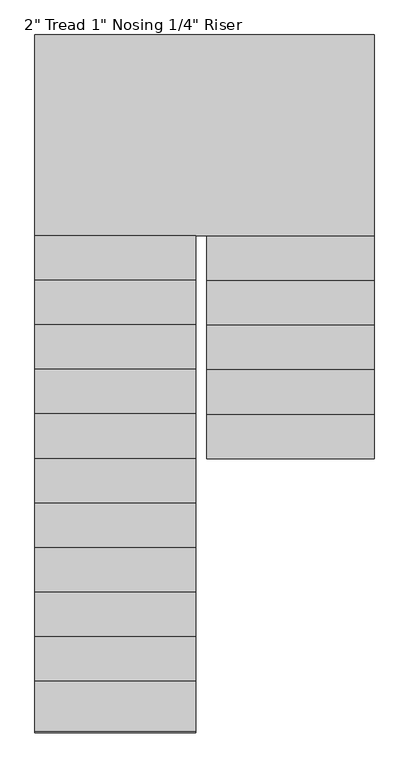
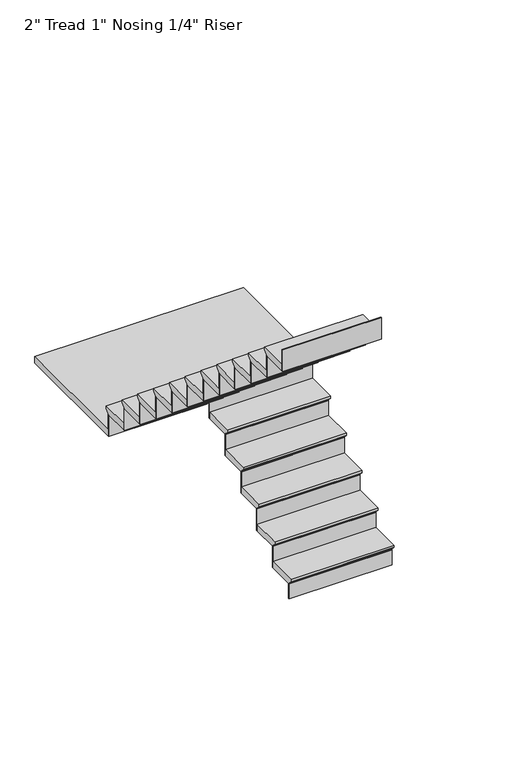
"""IFC4 building model written with IfcOpenShell, lengths in millimetres: stair flight geometry."""

from ifc_helpers import new_model, si_unit, origin, place, context, project, spatial, faceted_brep, source, transform, mapped, element, save


def stair_flight_b92ce0aa(model_context):
    return source(origin(), model_context, "Body", "Brep", [
        faceted_brep([(-3749.597125, 2714.6319226, 12189.8833333), (-3749.597125, 2714.6319226, 12208.9333333), (-4512.2136682, 2714.6319226, 12208.9333333), (-4512.2136682, 2714.6319226, 12189.8833333), (-3749.597125, 2740.0319226, 12164.4833333), (-4512.2136682, 2740.0319226, 12164.4833333), (-3749.597125, 2943.2319226, 12208.9333333), (-4512.2136682, 2943.2319226, 12208.9333333), (-4512.2136682, 2740.0319226, 12158.1333333), (-4512.2136682, 2943.2319226, 12158.1333333), (-3749.597125, 2943.2319226, 12158.1333333), (-3749.597125, 2740.0319226, 12158.1333333)], [[[0, 1, 2, 3]], [[4, 0, 3, 5]], [[2, 1, 6, 7]], [[8, 9, 10, 11]], [[2, 7, 9, 8, 5, 3]], [[8, 11, 4, 5]], [[6, 1, 0, 4, 11, 10]], [[7, 6, 10, 9]]]),
        faceted_brep([(-3749.597125, 2740.0319226, 12158.1333333), (-3749.597125, 2740.0319226, 12039.6), (-3749.597125, 2746.3819226, 12039.6), (-3749.597125, 2746.3819226, 12158.1333333), (-4512.2136682, 2740.0319226, 12158.1333333), (-4512.2136682, 2746.3819226, 12158.1333333), (-4512.2136682, 2746.3819226, 12039.6), (-4512.2136682, 2740.0319226, 12039.6)], [[[0, 1, 2, 3]], [[4, 5, 6, 7]], [[1, 0, 4, 7]], [[2, 1, 7, 6]], [[3, 2, 6, 5]], [[0, 3, 5, 4]]]),
        faceted_brep([(-3749.597125, 2943.2319226, 12327.4666667), (-3749.597125, 2943.2319226, 12158.1333333), (-3749.597125, 2949.5819226, 12158.1333333), (-3749.597125, 2949.5819226, 12327.4666667), (-4512.2136682, 2943.2319226, 12327.4666667), (-4512.2136682, 2949.5819226, 12327.4666667), (-4512.2136682, 2949.5819226, 12158.1333333), (-4512.2136682, 2943.2319226, 12158.1333333)], [[[0, 1, 2, 3]], [[4, 5, 6, 7]], [[1, 0, 4, 7]], [[2, 1, 7, 6]], [[3, 2, 6, 5]], [[0, 3, 5, 4]]]),
        faceted_brep([(-4512.2136682, 2917.8319226, 12378.2666667), (-3749.597125, 2917.8319226, 12378.2666667), (-3749.597125, 3146.4319226, 12378.2666667), (-4512.2136682, 3146.4319226, 12378.2666667), (-4512.2136682, 2943.2319226, 12327.4666667), (-4512.2136682, 3146.4319226, 12327.4666667), (-3749.597125, 3146.4319226, 12327.4666667), (-3749.597125, 2943.2319226, 12327.4666667), (-4512.2136682, 2943.2319226, 12333.8166667), (-4512.2136682, 2917.8319226, 12359.2166667), (-3749.597125, 2943.2319226, 12333.8166667), (-3749.597125, 2917.8319226, 12359.2166667)], [[[0, 1, 2, 3]], [[4, 5, 6, 7]], [[0, 3, 5, 4, 8, 9]], [[4, 7, 10, 8]], [[2, 1, 11, 10, 7, 6]], [[3, 2, 6, 5]], [[11, 1, 0, 9]], [[10, 11, 9, 8]]]),
        faceted_brep([(-3749.597125, 3146.4319226, 12496.8), (-3749.597125, 3146.4319226, 12327.4666667), (-3749.597125, 3152.7819226, 12327.4666667), (-3749.597125, 3152.7819226, 12496.8), (-4512.2136682, 3146.4319226, 12496.8), (-4512.2136682, 3152.7819226, 12496.8), (-4512.2136682, 3152.7819226, 12327.4666667), (-4512.2136682, 3146.4319226, 12327.4666667)], [[[0, 1, 2, 3]], [[4, 5, 6, 7]], [[1, 0, 4, 7]], [[2, 1, 7, 6]], [[3, 2, 6, 5]], [[0, 3, 5, 4]]]),
        faceted_brep([(-4512.2136682, 3121.0319226, 12547.6), (-3749.597125, 3121.0319226, 12547.6), (-3749.597125, 3349.6319226, 12547.6), (-4512.2136682, 3349.6319226, 12547.6), (-4512.2136682, 3146.4319226, 12496.8), (-4512.2136682, 3349.6319226, 12496.8), (-3749.597125, 3349.6319226, 12496.8), (-3749.597125, 3146.4319226, 12496.8), (-4512.2136682, 3146.4319226, 12503.15), (-4512.2136682, 3121.0319226, 12528.55), (-3749.597125, 3146.4319226, 12503.15), (-3749.597125, 3121.0319226, 12528.55)], [[[0, 1, 2, 3]], [[4, 5, 6, 7]], [[0, 3, 5, 4, 8, 9]], [[4, 7, 10, 8]], [[2, 1, 11, 10, 7, 6]], [[3, 2, 6, 5]], [[11, 1, 0, 9]], [[10, 11, 9, 8]]]),
        faceted_brep([(-3749.597125, 3349.6319226, 12666.1333333), (-3749.597125, 3349.6319226, 12496.8), (-3749.597125, 3355.9819226, 12496.8), (-3749.597125, 3355.9819226, 12666.1333333), (-4512.2136682, 3349.6319226, 12666.1333333), (-4512.2136682, 3355.9819226, 12666.1333333), (-4512.2136682, 3355.9819226, 12496.8), (-4512.2136682, 3349.6319226, 12496.8)], [[[0, 1, 2, 3]], [[4, 5, 6, 7]], [[1, 0, 4, 7]], [[2, 1, 7, 6]], [[3, 2, 6, 5]], [[0, 3, 5, 4]]]),
        faceted_brep([(-4512.2136682, 3324.2319226, 12716.9333333), (-3749.597125, 3324.2319226, 12716.9333333), (-3749.597125, 3552.8319226, 12716.9333333), (-4512.2136682, 3552.8319226, 12716.9333333), (-4512.2136682, 3349.6319226, 12666.1333333), (-4512.2136682, 3552.8319226, 12666.1333333), (-3749.597125, 3552.8319226, 12666.1333333), (-3749.597125, 3349.6319226, 12666.1333333), (-4512.2136682, 3349.6319226, 12672.4833333), (-4512.2136682, 3324.2319226, 12697.8833333), (-3749.597125, 3349.6319226, 12672.4833333), (-3749.597125, 3324.2319226, 12697.8833333)], [[[0, 1, 2, 3]], [[4, 5, 6, 7]], [[0, 3, 5, 4, 8, 9]], [[4, 7, 10, 8]], [[2, 1, 11, 10, 7, 6]], [[3, 2, 6, 5]], [[11, 1, 0, 9]], [[10, 11, 9, 8]]]),
        faceted_brep([(-3749.597125, 3552.8319226, 12835.4666667), (-3749.597125, 3552.8319226, 12666.1333333), (-3749.597125, 3559.1819226, 12666.1333333), (-3749.597125, 3559.1819226, 12835.4666667), (-4512.2136682, 3552.8319226, 12835.4666667), (-4512.2136682, 3559.1819226, 12835.4666667), (-4512.2136682, 3559.1819226, 12666.1333333), (-4512.2136682, 3552.8319226, 12666.1333333)], [[[0, 1, 2, 3]], [[4, 5, 6, 7]], [[1, 0, 4, 7]], [[2, 1, 7, 6]], [[3, 2, 6, 5]], [[0, 3, 5, 4]]]),
        faceted_brep([(-4512.2136682, 3527.4319226, 12886.2666667), (-3749.597125, 3527.4319226, 12886.2666667), (-3749.597125, 3756.0319226, 12886.2666667), (-4512.2136682, 3756.0319226, 12886.2666667), (-4512.2136682, 3552.8319226, 12835.4666667), (-4512.2136682, 3756.0319226, 12835.4666667), (-3749.597125, 3756.0319226, 12835.4666667), (-3749.597125, 3552.8319226, 12835.4666667), (-4512.2136682, 3552.8319226, 12841.8166667), (-4512.2136682, 3527.4319226, 12867.2166667), (-3749.597125, 3552.8319226, 12841.8166667), (-3749.597125, 3527.4319226, 12867.2166667)], [[[0, 1, 2, 3]], [[4, 5, 6, 7]], [[0, 3, 5, 4, 8, 9]], [[4, 7, 10, 8]], [[2, 1, 11, 10, 7, 6]], [[3, 2, 6, 5]], [[11, 1, 0, 9]], [[10, 11, 9, 8]]]),
        faceted_brep([(-3749.597125, 3756.0319226, 13004.8), (-3749.597125, 3756.0319226, 12835.4666667), (-3749.597125, 3762.3819226, 12835.4666667), (-3749.597125, 3762.3819226, 13004.8), (-4512.2136682, 3756.0319226, 13004.8), (-4512.2136682, 3762.3819226, 13004.8), (-4512.2136682, 3762.3819226, 12835.4666667), (-4512.2136682, 3756.0319226, 12835.4666667)], [[[0, 1, 2, 3]], [[4, 5, 6, 7]], [[1, 0, 4, 7]], [[2, 1, 7, 6]], [[3, 2, 6, 5]], [[0, 3, 5, 4]]]),
        faceted_brep([(-4563.0136682, 3705.2319226, 13055.6), (-4563.0136682, 3730.6319226, 13055.6), (-3749.597125, 3730.6319226, 13055.6), (-3749.597125, 4645.0319226, 13055.6), (-5295.0246464, 4645.0319226, 13055.6), (-5295.0246464, 3705.2319226, 13055.6), (-4563.0136682, 3730.6319226, 13004.8), (-4563.0136682, 3705.2319226, 13004.8), (-5295.0246464, 3705.2319226, 13004.8), (-5295.0246464, 4645.0319226, 13004.8), (-3749.597125, 4645.0319226, 13004.8), (-3749.597125, 3756.0319226, 13004.8), (-4512.2136682, 3756.0319226, 13004.8), (-4512.2136682, 3730.6319226, 13004.8), (-4512.2136682, 3730.6319226, 13036.55), (-3749.597125, 3730.6319226, 13036.55), (-4512.2136682, 3756.0319226, 13011.15), (-3749.597125, 3756.0319226, 13011.15)], [[[0, 1, 2, 3, 4, 5]], [[6, 7, 8, 9, 10, 11, 12, 13]], [[1, 0, 7, 6]], [[2, 1, 6, 13, 14, 15]], [[13, 12, 16, 14]], [[12, 11, 17, 16]], [[3, 2, 15, 17, 11, 10]], [[4, 3, 10, 9]], [[5, 4, 9, 8]], [[0, 5, 8, 7]], [[17, 15, 14, 16]]]),
        faceted_brep([(-5295.0246464, 3705.2319226, 13174.1333333), (-5295.0246464, 3705.2319226, 13004.8), (-5295.0246464, 3698.8819226, 13004.8), (-5295.0246464, 3698.8819226, 13174.1333333), (-4563.0136682, 3705.2319226, 13174.1333333), (-4563.0136682, 3698.8819226, 13174.1333333), (-4563.0136682, 3698.8819226, 13004.8), (-4563.0136682, 3705.2319226, 13004.8)], [[[0, 1, 2, 3]], [[4, 5, 6, 7]], [[1, 0, 4, 7]], [[2, 1, 7, 6]], [[3, 2, 6, 5]], [[0, 3, 5, 4]]]),
        faceted_brep([(-4563.0136682, 3730.6319226, 13224.9333333), (-5295.0246464, 3730.6319226, 13224.9333333), (-5295.0246464, 3502.0319226, 13224.9333333), (-4563.0136682, 3502.0319226, 13224.9333333), (-4563.0136682, 3705.2319226, 13174.1333333), (-4563.0136682, 3502.0319226, 13174.1333333), (-5295.0246464, 3502.0319226, 13174.1333333), (-5295.0246464, 3705.2319226, 13174.1333333), (-4563.0136682, 3705.2319226, 13180.4833333), (-4563.0136682, 3730.6319226, 13205.8833333), (-5295.0246464, 3705.2319226, 13180.4833333), (-5295.0246464, 3730.6319226, 13205.8833333)], [[[0, 1, 2, 3]], [[4, 5, 6, 7]], [[0, 3, 5, 4, 8, 9]], [[4, 7, 10, 8]], [[2, 1, 11, 10, 7, 6]], [[3, 2, 6, 5]], [[11, 1, 0, 9]], [[10, 11, 9, 8]]]),
        faceted_brep([(-5295.0246464, 3502.0319226, 13343.4666667), (-5295.0246464, 3502.0319226, 13174.1333333), (-5295.0246464, 3495.6819226, 13174.1333333), (-5295.0246464, 3495.6819226, 13343.4666667), (-4563.0136682, 3502.0319226, 13343.4666667), (-4563.0136682, 3495.6819226, 13343.4666667), (-4563.0136682, 3495.6819226, 13174.1333333), (-4563.0136682, 3502.0319226, 13174.1333333)], [[[0, 1, 2, 3]], [[4, 5, 6, 7]], [[1, 0, 4, 7]], [[2, 1, 7, 6]], [[3, 2, 6, 5]], [[0, 3, 5, 4]]]),
        faceted_brep([(-4563.0136682, 3527.4319226, 13394.2666667), (-5295.0246464, 3527.4319226, 13394.2666667), (-5295.0246464, 3298.8319226, 13394.2666667), (-4563.0136682, 3298.8319226, 13394.2666667), (-4563.0136682, 3502.0319226, 13343.4666667), (-4563.0136682, 3298.8319226, 13343.4666667), (-5295.0246464, 3298.8319226, 13343.4666667), (-5295.0246464, 3502.0319226, 13343.4666667), (-4563.0136682, 3502.0319226, 13349.8166667), (-4563.0136682, 3527.4319226, 13375.2166667), (-5295.0246464, 3502.0319226, 13349.8166667), (-5295.0246464, 3527.4319226, 13375.2166667)], [[[0, 1, 2, 3]], [[4, 5, 6, 7]], [[0, 3, 5, 4, 8, 9]], [[4, 7, 10, 8]], [[2, 1, 11, 10, 7, 6]], [[3, 2, 6, 5]], [[11, 1, 0, 9]], [[10, 11, 9, 8]]]),
        faceted_brep([(-5295.0246464, 3298.8319226, 13512.8), (-5295.0246464, 3298.8319226, 13343.4666667), (-5295.0246464, 3292.4819226, 13343.4666667), (-5295.0246464, 3292.4819226, 13512.8), (-4563.0136682, 3298.8319226, 13512.8), (-4563.0136682, 3292.4819226, 13512.8), (-4563.0136682, 3292.4819226, 13343.4666667), (-4563.0136682, 3298.8319226, 13343.4666667)], [[[0, 1, 2, 3]], [[4, 5, 6, 7]], [[1, 0, 4, 7]], [[2, 1, 7, 6]], [[3, 2, 6, 5]], [[0, 3, 5, 4]]]),
        faceted_brep([(-4563.0136682, 3324.2319226, 13563.6), (-5295.0246464, 3324.2319226, 13563.6), (-5295.0246464, 3095.6319226, 13563.6), (-4563.0136682, 3095.6319226, 13563.6), (-4563.0136682, 3298.8319226, 13512.8), (-4563.0136682, 3095.6319226, 13512.8), (-5295.0246464, 3095.6319226, 13512.8), (-5295.0246464, 3298.8319226, 13512.8), (-4563.0136682, 3298.8319226, 13519.15), (-4563.0136682, 3324.2319226, 13544.55), (-5295.0246464, 3298.8319226, 13519.15), (-5295.0246464, 3324.2319226, 13544.55)], [[[0, 1, 2, 3]], [[4, 5, 6, 7]], [[0, 3, 5, 4, 8, 9]], [[4, 7, 10, 8]], [[2, 1, 11, 10, 7, 6]], [[3, 2, 6, 5]], [[11, 1, 0, 9]], [[10, 11, 9, 8]]]),
        faceted_brep([(-5295.0246464, 3095.6319226, 13682.1333333), (-5295.0246464, 3095.6319226, 13512.8), (-5295.0246464, 3089.2819226, 13512.8), (-5295.0246464, 3089.2819226, 13682.1333333), (-4563.0136682, 3095.6319226, 13682.1333333), (-4563.0136682, 3089.2819226, 13682.1333333), (-4563.0136682, 3089.2819226, 13512.8), (-4563.0136682, 3095.6319226, 13512.8)], [[[0, 1, 2, 3]], [[4, 5, 6, 7]], [[1, 0, 4, 7]], [[2, 1, 7, 6]], [[3, 2, 6, 5]], [[0, 3, 5, 4]]]),
        faceted_brep([(-4563.0136682, 3121.0319226, 13732.9333333), (-5295.0246464, 3121.0319226, 13732.9333333), (-5295.0246464, 2892.4319226, 13732.9333333), (-4563.0136682, 2892.4319226, 13732.9333333), (-4563.0136682, 3095.6319226, 13682.1333333), (-4563.0136682, 2892.4319226, 13682.1333333), (-5295.0246464, 2892.4319226, 13682.1333333), (-5295.0246464, 3095.6319226, 13682.1333333), (-4563.0136682, 3095.6319226, 13688.4833333), (-4563.0136682, 3121.0319226, 13713.8833333), (-5295.0246464, 3095.6319226, 13688.4833333), (-5295.0246464, 3121.0319226, 13713.8833333)], [[[0, 1, 2, 3]], [[4, 5, 6, 7]], [[0, 3, 5, 4, 8, 9]], [[4, 7, 10, 8]], [[2, 1, 11, 10, 7, 6]], [[3, 2, 6, 5]], [[11, 1, 0, 9]], [[10, 11, 9, 8]]]),
        faceted_brep([(-5295.0246464, 2892.4319226, 13851.4666667), (-5295.0246464, 2892.4319226, 13682.1333333), (-5295.0246464, 2886.0819226, 13682.1333333), (-5295.0246464, 2886.0819226, 13851.4666667), (-4563.0136682, 2892.4319226, 13851.4666667), (-4563.0136682, 2886.0819226, 13851.4666667), (-4563.0136682, 2886.0819226, 13682.1333333), (-4563.0136682, 2892.4319226, 13682.1333333)], [[[0, 1, 2, 3]], [[4, 5, 6, 7]], [[1, 0, 4, 7]], [[2, 1, 7, 6]], [[3, 2, 6, 5]], [[0, 3, 5, 4]]]),
        faceted_brep([(-4563.0136682, 2917.8319226, 13902.2666667), (-5295.0246464, 2917.8319226, 13902.2666667), (-5295.0246464, 2689.2319226, 13902.2666667), (-4563.0136682, 2689.2319226, 13902.2666667), (-4563.0136682, 2892.4319226, 13851.4666667), (-4563.0136682, 2689.2319226, 13851.4666667), (-5295.0246464, 2689.2319226, 13851.4666667), (-5295.0246464, 2892.4319226, 13851.4666667), (-4563.0136682, 2892.4319226, 13857.8166667), (-4563.0136682, 2917.8319226, 13883.2166667), (-5295.0246464, 2892.4319226, 13857.8166667), (-5295.0246464, 2917.8319226, 13883.2166667)], [[[0, 1, 2, 3]], [[4, 5, 6, 7]], [[0, 3, 5, 4, 8, 9]], [[4, 7, 10, 8]], [[2, 1, 11, 10, 7, 6]], [[3, 2, 6, 5]], [[11, 1, 0, 9]], [[10, 11, 9, 8]]]),
        faceted_brep([(-5295.0246464, 2689.2319226, 14020.8), (-5295.0246464, 2689.2319226, 13851.4666667), (-5295.0246464, 2682.8819226, 13851.4666667), (-5295.0246464, 2682.8819226, 14020.8), (-4563.0136682, 2689.2319226, 14020.8), (-4563.0136682, 2682.8819226, 14020.8), (-4563.0136682, 2682.8819226, 13851.4666667), (-4563.0136682, 2689.2319226, 13851.4666667)], [[[0, 1, 2, 3]], [[4, 5, 6, 7]], [[1, 0, 4, 7]], [[2, 1, 7, 6]], [[3, 2, 6, 5]], [[0, 3, 5, 4]]]),
        faceted_brep([(-4563.0136682, 2714.6319226, 14071.6), (-5295.0246464, 2714.6319226, 14071.6), (-5295.0246464, 2486.0319226, 14071.6), (-4563.0136682, 2486.0319226, 14071.6), (-4563.0136682, 2689.2319226, 14020.8), (-4563.0136682, 2486.0319226, 14020.8), (-5295.0246464, 2486.0319226, 14020.8), (-5295.0246464, 2689.2319226, 14020.8), (-4563.0136682, 2689.2319226, 14027.15), (-4563.0136682, 2714.6319226, 14052.55), (-5295.0246464, 2689.2319226, 14027.15), (-5295.0246464, 2714.6319226, 14052.55)], [[[0, 1, 2, 3]], [[4, 5, 6, 7]], [[0, 3, 5, 4, 8, 9]], [[4, 7, 10, 8]], [[2, 1, 11, 10, 7, 6]], [[3, 2, 6, 5]], [[11, 1, 0, 9]], [[10, 11, 9, 8]]]),
        faceted_brep([(-5295.0246464, 2486.0319226, 14190.1333333), (-5295.0246464, 2486.0319226, 14020.8), (-5295.0246464, 2479.6819226, 14020.8), (-5295.0246464, 2479.6819226, 14190.1333333), (-4563.0136682, 2486.0319226, 14190.1333333), (-4563.0136682, 2479.6819226, 14190.1333333), (-4563.0136682, 2479.6819226, 14020.8), (-4563.0136682, 2486.0319226, 14020.8)], [[[0, 1, 2, 3]], [[4, 5, 6, 7]], [[1, 0, 4, 7]], [[2, 1, 7, 6]], [[3, 2, 6, 5]], [[0, 3, 5, 4]]]),
        faceted_brep([(-4563.0136682, 2511.4319226, 14240.9333333), (-5295.0246464, 2511.4319226, 14240.9333333), (-5295.0246464, 2282.8319226, 14240.9333333), (-4563.0136682, 2282.8319226, 14240.9333333), (-4563.0136682, 2486.0319226, 14190.1333333), (-4563.0136682, 2282.8319226, 14190.1333333), (-5295.0246464, 2282.8319226, 14190.1333333), (-5295.0246464, 2486.0319226, 14190.1333333), (-4563.0136682, 2486.0319226, 14196.4833333), (-4563.0136682, 2511.4319226, 14221.8833333), (-5295.0246464, 2486.0319226, 14196.4833333), (-5295.0246464, 2511.4319226, 14221.8833333)], [[[0, 1, 2, 3]], [[4, 5, 6, 7]], [[0, 3, 5, 4, 8, 9]], [[4, 7, 10, 8]], [[2, 1, 11, 10, 7, 6]], [[3, 2, 6, 5]], [[11, 1, 0, 9]], [[10, 11, 9, 8]]]),
        faceted_brep([(-5295.0246464, 2282.8319226, 14359.4666667), (-5295.0246464, 2282.8319226, 14190.1333333), (-5295.0246464, 2276.4819226, 14190.1333333), (-5295.0246464, 2276.4819226, 14359.4666667), (-4563.0136682, 2282.8319226, 14359.4666667), (-4563.0136682, 2276.4819226, 14359.4666667), (-4563.0136682, 2276.4819226, 14190.1333333), (-4563.0136682, 2282.8319226, 14190.1333333)], [[[0, 1, 2, 3]], [[4, 5, 6, 7]], [[1, 0, 4, 7]], [[2, 1, 7, 6]], [[3, 2, 6, 5]], [[0, 3, 5, 4]]]),
        faceted_brep([(-4563.0136682, 2308.2319226, 14410.2666667), (-5295.0246464, 2308.2319226, 14410.2666667), (-5295.0246464, 2079.6319226, 14410.2666667), (-4563.0136682, 2079.6319226, 14410.2666667), (-4563.0136682, 2282.8319226, 14359.4666667), (-4563.0136682, 2079.6319226, 14359.4666667), (-5295.0246464, 2079.6319226, 14359.4666667), (-5295.0246464, 2282.8319226, 14359.4666667), (-4563.0136682, 2282.8319226, 14365.8166667), (-4563.0136682, 2308.2319226, 14391.2166667), (-5295.0246464, 2282.8319226, 14365.8166667), (-5295.0246464, 2308.2319226, 14391.2166667)], [[[0, 1, 2, 3]], [[4, 5, 6, 7]], [[0, 3, 5, 4, 8, 9]], [[4, 7, 10, 8]], [[2, 1, 11, 10, 7, 6]], [[3, 2, 6, 5]], [[11, 1, 0, 9]], [[10, 11, 9, 8]]]),
        faceted_brep([(-5295.0246464, 2079.6319226, 14528.8), (-5295.0246464, 2079.6319226, 14359.4666667), (-5295.0246464, 2073.2819226, 14359.4666667), (-5295.0246464, 2073.2819226, 14528.8), (-4563.0136682, 2079.6319226, 14528.8), (-4563.0136682, 2073.2819226, 14528.8), (-4563.0136682, 2073.2819226, 14359.4666667), (-4563.0136682, 2079.6319226, 14359.4666667)], [[[0, 1, 2, 3]], [[4, 5, 6, 7]], [[1, 0, 4, 7]], [[2, 1, 7, 6]], [[3, 2, 6, 5]], [[0, 3, 5, 4]]]),
        faceted_brep([(-4563.0136682, 2105.0319226, 14579.6), (-5295.0246464, 2105.0319226, 14579.6), (-5295.0246464, 1876.4319226, 14579.6), (-4563.0136682, 1876.4319226, 14579.6), (-4563.0136682, 2079.6319226, 14528.8), (-4563.0136682, 1876.4319226, 14528.8), (-5295.0246464, 1876.4319226, 14528.8), (-5295.0246464, 2079.6319226, 14528.8), (-4563.0136682, 2079.6319226, 14535.15), (-4563.0136682, 2105.0319226, 14560.55), (-5295.0246464, 2079.6319226, 14535.15), (-5295.0246464, 2105.0319226, 14560.55)], [[[0, 1, 2, 3]], [[4, 5, 6, 7]], [[0, 3, 5, 4, 8, 9]], [[4, 7, 10, 8]], [[2, 1, 11, 10, 7, 6]], [[3, 2, 6, 5]], [[11, 1, 0, 9]], [[10, 11, 9, 8]]]),
        faceted_brep([(-5295.0246464, 1876.4319226, 14698.1333333), (-5295.0246464, 1876.4319226, 14528.8), (-5295.0246464, 1870.0819226, 14528.8), (-5295.0246464, 1870.0819226, 14698.1333333), (-4563.0136682, 1876.4319226, 14698.1333333), (-4563.0136682, 1870.0819226, 14698.1333333), (-4563.0136682, 1870.0819226, 14528.8), (-4563.0136682, 1876.4319226, 14528.8)], [[[0, 1, 2, 3]], [[4, 5, 6, 7]], [[1, 0, 4, 7]], [[2, 1, 7, 6]], [[3, 2, 6, 5]], [[0, 3, 5, 4]]]),
        faceted_brep([(-4563.0136682, 1901.8319226, 14748.9333333), (-5295.0246464, 1901.8319226, 14748.9333333), (-5295.0246464, 1673.2319226, 14748.9333333), (-4563.0136682, 1673.2319226, 14748.9333333), (-4563.0136682, 1876.4319226, 14698.1333333), (-4563.0136682, 1673.2319226, 14698.1333333), (-5295.0246464, 1673.2319226, 14698.1333333), (-5295.0246464, 1876.4319226, 14698.1333333), (-4563.0136682, 1876.4319226, 14704.4833333), (-4563.0136682, 1901.8319226, 14729.8833333), (-5295.0246464, 1876.4319226, 14704.4833333), (-5295.0246464, 1901.8319226, 14729.8833333)], [[[0, 1, 2, 3]], [[4, 5, 6, 7]], [[0, 3, 5, 4, 8, 9]], [[4, 7, 10, 8]], [[2, 1, 11, 10, 7, 6]], [[3, 2, 6, 5]], [[11, 1, 0, 9]], [[10, 11, 9, 8]]]),
        faceted_brep([(-5295.0246464, 1673.2319226, 14867.4666667), (-5295.0246464, 1673.2319226, 14698.1333333), (-5295.0246464, 1666.8819226, 14698.1333333), (-5295.0246464, 1666.8819226, 14867.4666667), (-4563.0136682, 1673.2319226, 14867.4666667), (-4563.0136682, 1666.8819226, 14867.4666667), (-4563.0136682, 1666.8819226, 14698.1333333), (-4563.0136682, 1673.2319226, 14698.1333333)], [[[0, 1, 2, 3]], [[4, 5, 6, 7]], [[1, 0, 4, 7]], [[2, 1, 7, 6]], [[3, 2, 6, 5]], [[0, 3, 5, 4]]]),
        faceted_brep([(-4563.0136682, 1698.6319226, 14918.2666667), (-5295.0246464, 1698.6319226, 14918.2666667), (-5295.0246464, 1470.0319226, 14918.2666667), (-4563.0136682, 1470.0319226, 14918.2666667), (-4563.0136682, 1673.2319226, 14867.4666667), (-4563.0136682, 1470.0319226, 14867.4666667), (-5295.0246464, 1470.0319226, 14867.4666667), (-5295.0246464, 1673.2319226, 14867.4666667), (-4563.0136682, 1673.2319226, 14873.8166667), (-4563.0136682, 1698.6319226, 14899.2166667), (-5295.0246464, 1673.2319226, 14873.8166667), (-5295.0246464, 1698.6319226, 14899.2166667)], [[[0, 1, 2, 3]], [[4, 5, 6, 7]], [[0, 3, 5, 4, 8, 9]], [[4, 7, 10, 8]], [[2, 1, 11, 10, 7, 6]], [[3, 2, 6, 5]], [[11, 1, 0, 9]], [[10, 11, 9, 8]]]),
        faceted_brep([(-5295.0246464, 1470.0319226, 15036.8), (-5295.0246464, 1470.0319226, 14867.4666667), (-5295.0246464, 1463.6819226, 14867.4666667), (-5295.0246464, 1463.6819226, 15036.8), (-4563.0136682, 1470.0319226, 15036.8), (-4563.0136682, 1463.6819226, 15036.8), (-4563.0136682, 1463.6819226, 14867.4666667), (-4563.0136682, 1470.0319226, 14867.4666667)], [[[0, 1, 2, 3]], [[4, 5, 6, 7]], [[1, 0, 4, 7]], [[2, 1, 7, 6]], [[3, 2, 6, 5]], [[0, 3, 5, 4]]]),
    ])


if __name__ == "__main__":
    model = new_model("IFC4")
    model_context = context("Model", 3, world=origin())
    ifc_project = project(units=[si_unit("LENGTHUNIT", "METRE", prefix="MILLI")], contexts=[model_context])
    site = spatial("IfcSite", under=ifc_project)
    building = spatial("IfcBuilding", under=site)
    placement = place(None, origin())
    stair_flight_shape = stair_flight_b92ce0aa(model_context)
    element("IfcStairFlight", 1, ObjectType="2\" Tread 1\" Nosing 1/4\" Riser", at=placement, inside=building, context=model_context, shape_type="MappedRepresentation", body=[
        mapped(stair_flight_shape, transform((0.0, 0.0, 0.0), x_axis=(1.0, 0.0, 0.0), y_axis=(0.0, 1.0, 0.0), z_axis=(0.0, 0.0, 1.0))),
    ])
    save(model, "model.ifc")
